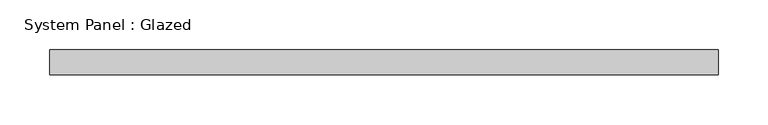
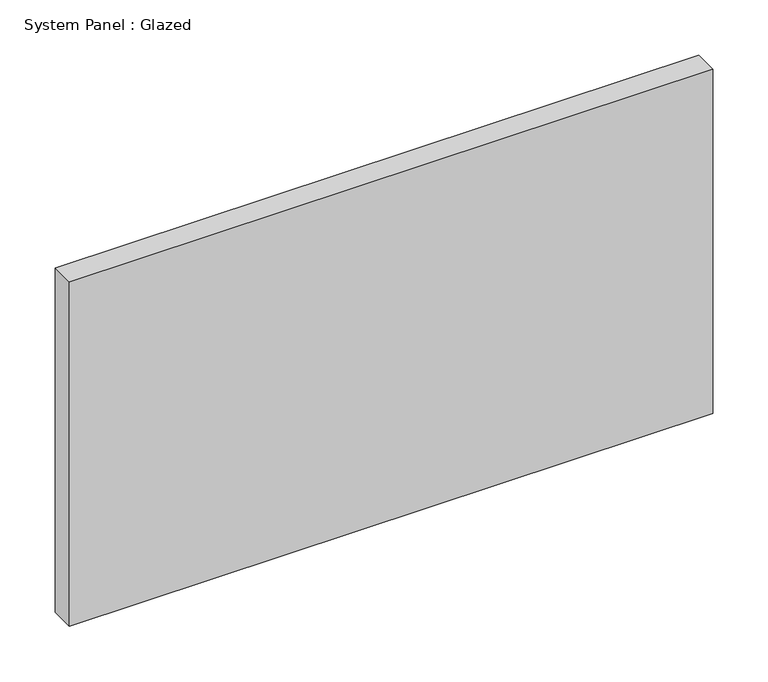
"""IFC4 building model written with IfcOpenShell, lengths in millimetres: plate geometry, System Panel : Glazed."""

from ifc_helpers import new_model, si_unit, origin, origin_with_axes, place, context, project, spatial, polyline, outline, extrude, source, transform, mapped, element, save


def system_panel_glazed_d62326f9(model_context):
    return source(origin(), model_context, "Body", "SweptSolid", [
        extrude(outline(polyline([(336.55, 19.05), (-336.55, 19.05), (-336.55, 44.45), (336.55, 44.45), (336.55, 19.05)])), origin_with_axes(), (0.0, 0.0, 1.0), 381.0),
    ])


if __name__ == "__main__":
    model = new_model("IFC4")
    model_context = context("Model", 3, world=origin())
    ifc_project = project(units=[si_unit("LENGTHUNIT", "METRE", prefix="MILLI")], contexts=[model_context])
    site = spatial("IfcSite", under=ifc_project)
    building = spatial("IfcBuilding", under=site)
    placement = place(None, origin())
    system_panel_glazed_shape = system_panel_glazed_d62326f9(model_context)
    element("IfcPlate", 1, ObjectType="System Panel : Glazed", at=placement, inside=building, context=model_context, shape_type="MappedRepresentation", body=[
        mapped(system_panel_glazed_shape, transform((0.0, 0.0, 0.0), x_axis=(1.0, 0.0, 0.0), y_axis=(0.0, 1.0, 0.0), z_axis=(0.0, 0.0, 1.0))),
    ])
    save(model, "model.ifc")

# Revit data of these elements
# Type "System Panel : Glazed"
#   Construction Type Id = "GSP4R"
#   Analytic Construction = "1/8 in Pilkington single glazing"
#   Visual Light Transmittance = 0.9
#   Solar Heat Gain Coefficient = 0.86
#   Heat Transfer Coefficient (U) = 1.18115 BTU/(h·ft²·°F)
#   Define Thermal Properties by = 1
# Element 1 (IfcPlate, "System Panel : Glazed")
#   Materials on its faces: "Glass"
# Materials
#   "Glass": class "Glass", colour RGB 0 128 192, transparency 0.75, Description = "Soda Lime Glass", Cost = 0
